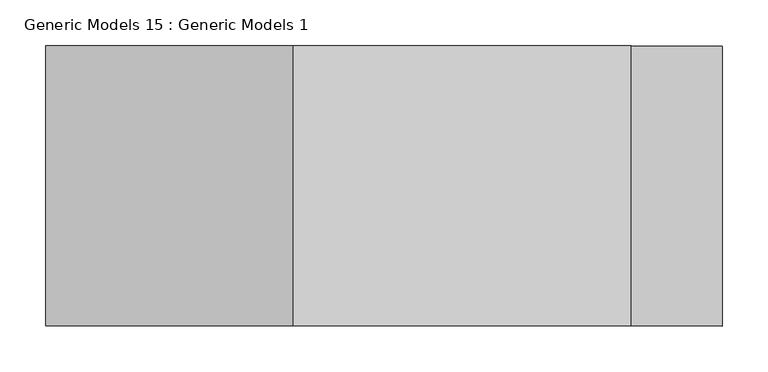
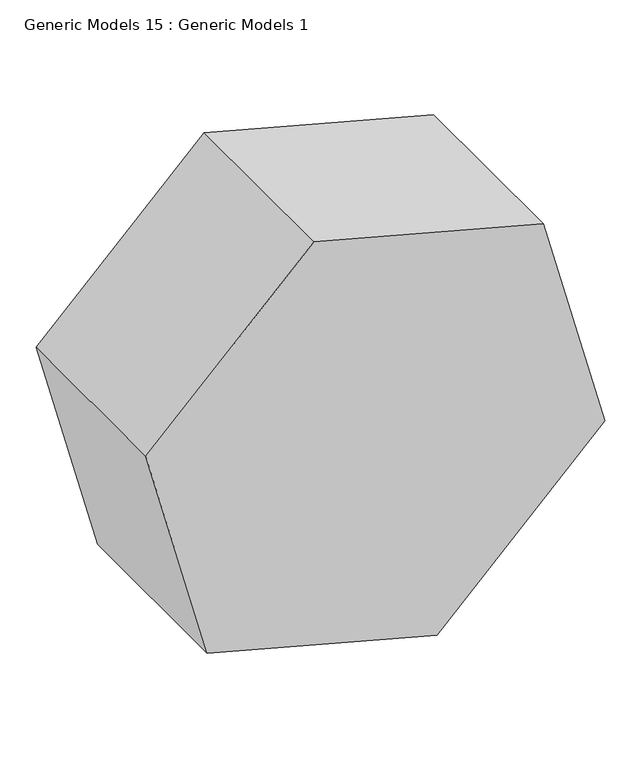
"""IFC4 building model written with IfcOpenShell, lengths in millimetres: proxy geometry, Generic Models 15 : Generic Models 1."""

from ifc_helpers import new_model, si_unit, frame, origin, place, context, project, spatial, polyline, outline, extrude, source, transform, mapped, element, save


def generic_models_15_generic_models_1_a1369ee7(model_context):
    return source(origin(), model_context, "Body", "SweptSolid", [
        extrude(outline(polyline([(904.7566299, 6078.6198357), (1003.366686, 5710.6020959), (733.9590024, 5441.1944123), (365.9412626, 5539.8044685), (267.3312064, 5907.8222083), (536.73889, 6177.2298919), (904.7566299, 6078.6198357)])), frame((0.0, -9086.6225464, 0.0), z_axis=(0.0, 1.0, 0.0), x_axis=(0.0, 0.0, 1.0)), (0.0, 0.0, 1.0), 304.8),
    ])


if __name__ == "__main__":
    model = new_model("IFC4")
    model_context = context("Model", 3, world=origin())
    ifc_project = project(units=[si_unit("LENGTHUNIT", "METRE", prefix="MILLI")], contexts=[model_context])
    site = spatial("IfcSite", under=ifc_project)
    building = spatial("IfcBuilding", under=site)
    placement = place(None, origin())
    generic_models_15_generic_models_1_shape = generic_models_15_generic_models_1_a1369ee7(model_context)
    element("IfcBuildingElementProxy", 1, Name="Generic Models 15 : Generic Models 1", ObjectType="Generic Models 15 : Generic Models 1", at=placement, inside=building, context=model_context, shape_type="MappedRepresentation", body=[
        mapped(generic_models_15_generic_models_1_shape, transform((0.0, 0.0, 0.0), x_axis=(1.0, 0.0, 0.0), y_axis=(0.0, 1.0, 0.0), z_axis=(0.0, 0.0, 1.0))),
    ])
    save(model, "model.ifc")

# Revit data of these elements
# Element 1 (IfcBuildingElementProxy, "Generic Models 15 : Generic Models 1")
#   Materials on its faces: "Carpet (1)"
# Materials
#   "Carpet (1)": class "Carpet", colour RGB 124 80 67, transparency 0, Description = "Interior finish", Cost = 0
